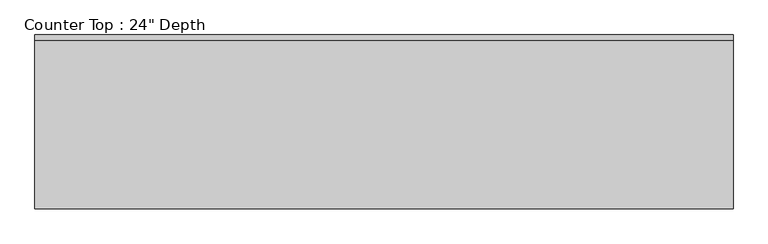
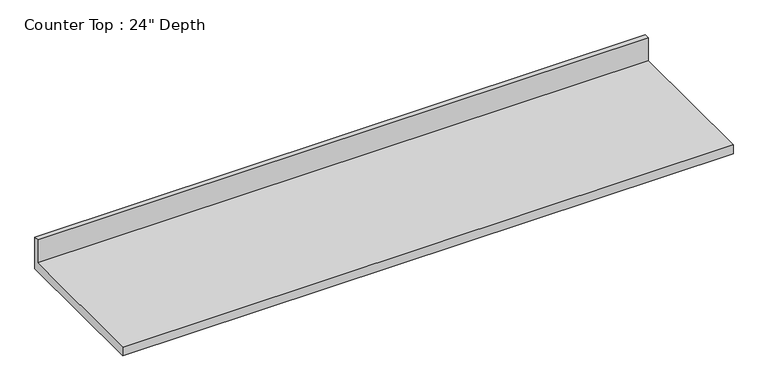
"""IFC4 building model written with IfcOpenShell, lengths in millimetres: furniture geometry."""

from ifc_helpers import new_model, si_unit, frame, origin, place, context, project, spatial, polyline, outline, extrude, source, transform, mapped, element, save


def furniture_0b9e3d50(model_context):
    return source(origin(), model_context, "Body", "SweptSolid", [
        extrude(outline(polyline([(0.0, 1016.0), (0.0, 876.3), (-635.0, 876.3), (-635.0, 914.4), (-19.05, 914.4), (-19.05, 1016.0), (0.0, 1016.0)])), frame((-1200.4622951, 0.0, 0.0), z_axis=(1.0, 0.0, 0.0), x_axis=(0.0, 1.0, 0.0)), (0.0, 0.0, 1.0), 2552.7),
    ])


if __name__ == "__main__":
    model = new_model("IFC4")
    model_context = context("Model", 3, world=origin())
    ifc_project = project(units=[si_unit("LENGTHUNIT", "METRE", prefix="MILLI")], contexts=[model_context])
    site = spatial("IfcSite", under=ifc_project)
    building = spatial("IfcBuilding", under=site)
    placement = place(None, origin())
    furniture_shape = furniture_0b9e3d50(model_context)
    element("IfcFurniture", 1, ObjectType="Counter Top : 24\" Depth", at=placement, inside=building, context=model_context, shape_type="MappedRepresentation", body=[
        mapped(furniture_shape, transform((0.0, 0.0, 0.0), x_axis=(1.0, 0.0, 0.0), y_axis=(0.0, 1.0, 0.0), z_axis=(0.0, 0.0, 1.0))),
    ])
    save(model, "model.ifc")

# Revit data of these elements
# Type "Counter Top : 24\" Depth"
#   Assembly Code = "C1030400"
#   Counter Thickness = 0' - 1 1/2"
#   Depth = 2' - 1"
#   Height = 3' - 0"
#   Length [instance default] = 8' - 0"
#   Counter Top Material = none
#   Default Elevation = 0
# Element 1 (IfcFurniture, "Counter Top : 24\" Depth")
#   Length = 8' - 4 1/2"
#   Materials on its faces: "Counter Top"
# Materials
#   "Counter Top": class "Wood", colour RGB 226 177 128, transparency 0
